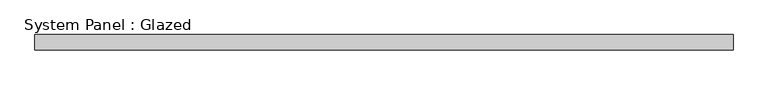
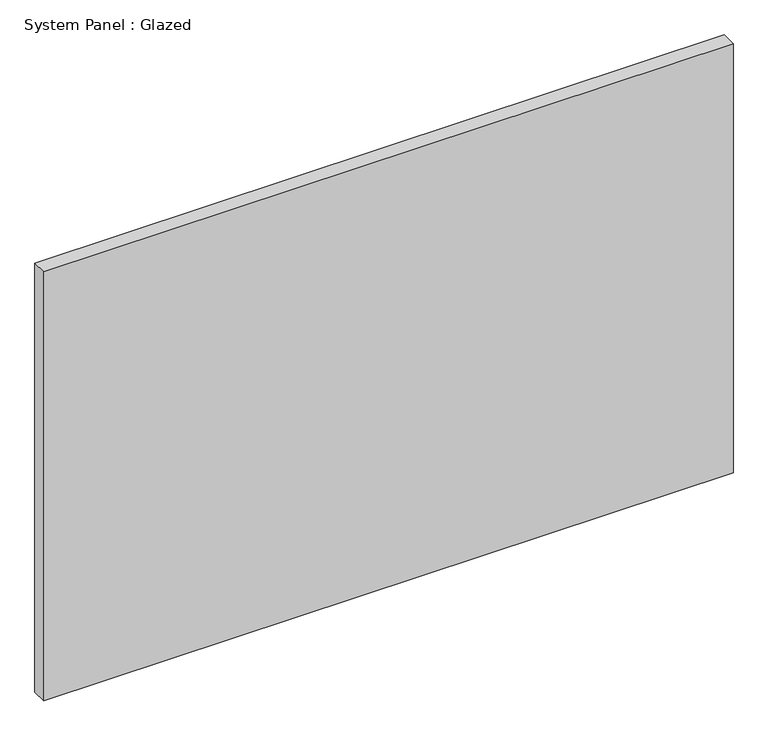
"""IFC4 building model written with IfcOpenShell, lengths in millimetres: plate geometry, System Panel : Glazed."""

from ifc_helpers import new_model, si_unit, origin, origin_with_axes, place, context, project, spatial, polyline, outline, extrude, source, transform, mapped, element, save


def system_panel_glazed_6fb9d5dc(model_context):
    return source(origin(), model_context, "Body", "SweptSolid", [
        extrude(outline(polyline([(577.693898, 19.05), (-577.693898, 19.05), (-577.693898, 44.45), (577.693898, 44.45), (577.693898, 19.05)])), origin_with_axes(), (0.0, 0.0, 1.0), 760.0438093),
    ])


if __name__ == "__main__":
    model = new_model("IFC4")
    model_context = context("Model", 3, world=origin())
    ifc_project = project(units=[si_unit("LENGTHUNIT", "METRE", prefix="MILLI")], contexts=[model_context])
    site = spatial("IfcSite", under=ifc_project)
    building = spatial("IfcBuilding", under=site)
    placement = place(None, origin())
    system_panel_glazed_shape = system_panel_glazed_6fb9d5dc(model_context)
    element("IfcPlate", 1, ObjectType="System Panel : Glazed", at=placement, inside=building, context=model_context, shape_type="MappedRepresentation", body=[
        mapped(system_panel_glazed_shape, transform((0.0, 0.0, 0.0), x_axis=(1.0, 0.0, 0.0), y_axis=(0.0, 1.0, 0.0), z_axis=(0.0, 0.0, 1.0))),
    ])
    save(model, "model.ifc")

# Revit data of these elements
# Type "System Panel : Glazed"
#   Construction Type Id = "GSP4R"
#   Analytic Construction = "1/8 in Pilkington single glazing"
#   Visual Light Transmittance = 0.9
#   Solar Heat Gain Coefficient = 0.86
#   Heat Transfer Coefficient (U) = 1.18115 BTU/(h·ft²·°F)
#   Define Thermal Properties by = 1
# Element 1 (IfcPlate, "System Panel : Glazed")
#   Materials on its faces: "Glass"
# Materials
#   "Glass": class "Glass", colour RGB 0 128 192, transparency 0.75, Description = "Soda Lime Glass", Cost = 0
